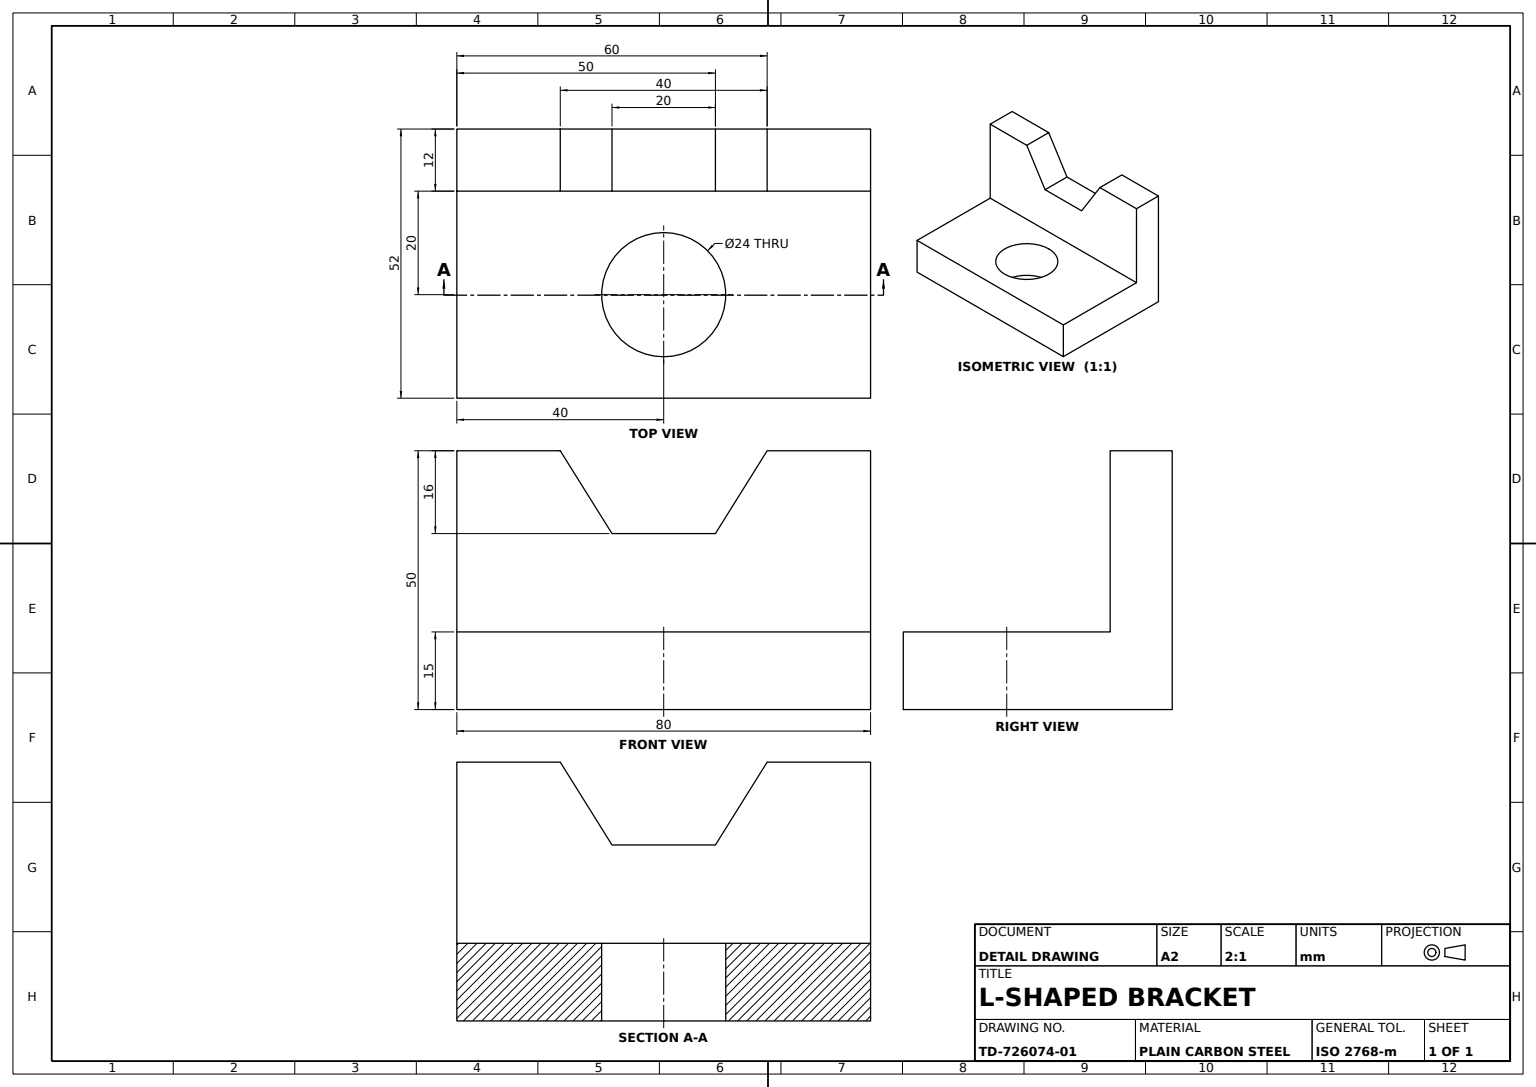
from build123d import *

# Parameters (mm, degrees)
UPRIGHT_V_NOTCH_PLATE_DEPTH = 12
BASE_PLATE_SKETCH_W         = 80
BASE_PLATE_SKETCH_H         = 15
BASE_PLATE_DEPTH            = 40
BASE_HOLE_SKETCH_24_R       = 12
BASE_HOLE_24_DEPTH          = 20


with BuildPart() as part:
    # Upright V-Notch Profile Sketch → Upright V-Notch Plate (new body)
    with BuildSketch(Plane.XY):
        Polygon((0, 0), (0, -50), (80, -50), (80, 0), (60, 0), (50, -16), (30, -16), (20, 0), align=None)
    extrude(amount=UPRIGHT_V_NOTCH_PLATE_DEPTH)

    # Base Plate Sketch → Base Plate (add)
    with BuildSketch(Plane.XY.offset(12)):
        with Locations((40, -42.5)):
            Rectangle(BASE_PLATE_SKETCH_W, BASE_PLATE_SKETCH_H)
    extrude(amount=BASE_PLATE_DEPTH)

    # Base Hole Sketch Ø24 → Base Hole Ø24 (cut)
    with BuildSketch(Plane(origin=(0, -35, 0), x_dir=(1, 0, 0), z_dir=(0, 1, 0))):
        with Locations(Location((40, -32, 0), (0, 0, 270))):
            Circle(BASE_HOLE_SKETCH_24_R)
    extrude(amount=-BASE_HOLE_24_DEPTH, mode=Mode.SUBTRACT)


solid = part.part
